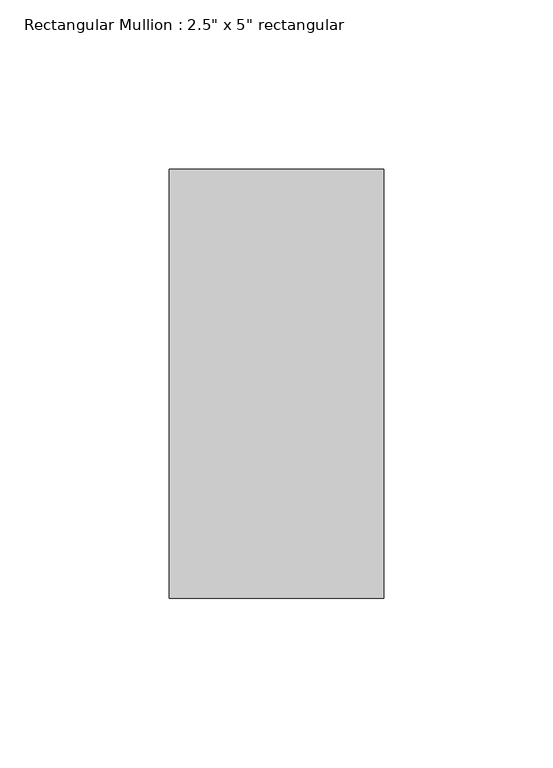
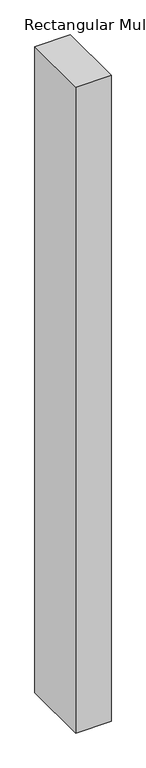
"""IFC4 building model written with IfcOpenShell, lengths in millimetres: member geometry."""

from ifc_helpers import new_model, si_unit, frame, origin, place, context, project, spatial, polyline, outline, extrude, source, transform, mapped, element, save


def member_65ceef43(model_context):
    return source(origin(), model_context, "Body", "SweptSolid", [
        extrude(outline(polyline([(31.75, 63.5), (31.75, -63.5), (-31.75, -63.5), (-31.75, 63.5), (31.75, 63.5)])), frame((0.0, 0.0, -1226.8199999), z_axis=(0.0, 0.0, 1.0), x_axis=(1.0, 0.0, 0.0)), (0.0, 0.0, 1.0), 1226.8199999),
    ])


if __name__ == "__main__":
    model = new_model("IFC4")
    model_context = context("Model", 3, world=origin())
    ifc_project = project(units=[si_unit("LENGTHUNIT", "METRE", prefix="MILLI")], contexts=[model_context])
    site = spatial("IfcSite", under=ifc_project)
    building = spatial("IfcBuilding", under=site)
    placement = place(None, origin())
    member_shape = member_65ceef43(model_context)
    element("IfcMember", 1, ObjectType="Rectangular Mullion : 2.5\" x 5\" rectangular", at=placement, inside=building, context=model_context, shape_type="MappedRepresentation", body=[
        mapped(member_shape, transform((0.0, 0.0, 0.0), x_axis=(1.0, 0.0, 0.0), y_axis=(0.0, 1.0, 0.0), z_axis=(0.0, 0.0, 1.0))),
    ])
    save(model, "model.ifc")

# Revit data of these elements
# Type "Rectangular Mullion : 2.5\" x 5\" rectangular"
#   built-in parameter 1007304 = 0.416667 (stored number, unit not read)
#   built-in parameter 1007301 = 0.104167 (stored number, unit not read)
#   built-in parameter 1007300 = 0.104167 (stored number, unit not read)
# Element 1 (IfcMember, "Rectangular Mullion : 2.5\" x 5\" rectangular")
#   Materials on its faces: "BLACK COLOUR"
# Materials
#   "BLACK COLOUR": class "Generic", colour RGB 120 120 120, transparency 0, Cost = 0
